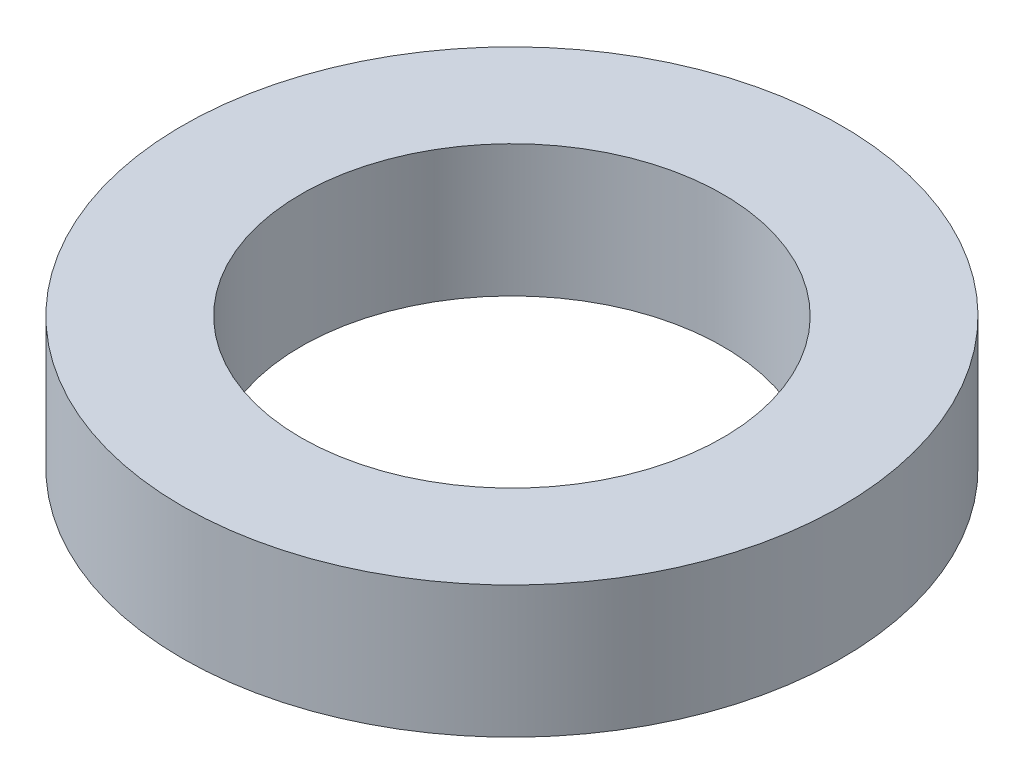
ISO-10303-21;
HEADER;
FILE_DESCRIPTION(('STEP AP214'),'2;1');
FILE_NAME('part.step','',(''),(''),'','','');
FILE_SCHEMA(('AUTOMOTIVE_DESIGN { 1 0 10303 214 1 1 1 1 }'));
ENDSEC;
DATA;
#1=APPLICATION_CONTEXT('core data for automotive mechanical design processes');
#2=APPLICATION_PROTOCOL_DEFINITION('international standard','automotive_design',2000,#1);
#3=PRODUCT_CONTEXT('',#1,'mechanical');
#4=PRODUCT('Part','Part','',(#3));
#5=PRODUCT_RELATED_PRODUCT_CATEGORY('part','',(#4));
#6=PRODUCT_DEFINITION_FORMATION('','',#4);
#7=PRODUCT_DEFINITION_CONTEXT('part definition',#1,'design');
#8=PRODUCT_DEFINITION('design','',#6,#7);
#9=PRODUCT_DEFINITION_SHAPE('','',#8);
#10=(LENGTH_UNIT() NAMED_UNIT(*) SI_UNIT(.MILLI.,.METRE.));
#11=(NAMED_UNIT(*) PLANE_ANGLE_UNIT() SI_UNIT($,.RADIAN.));
#12=(NAMED_UNIT(*) SI_UNIT($,.STERADIAN.) SOLID_ANGLE_UNIT());
#13=UNCERTAINTY_MEASURE_WITH_UNIT(LENGTH_MEASURE(1.E-05),#10,'distance_accuracy_value','');
#14=(GEOMETRIC_REPRESENTATION_CONTEXT(3) GLOBAL_UNCERTAINTY_ASSIGNED_CONTEXT((#13)) GLOBAL_UNIT_ASSIGNED_CONTEXT((#10,
#11,#12)) REPRESENTATION_CONTEXT('',''));
#15=CARTESIAN_POINT('',(0.,0.,0.));
#16=DIRECTION('',(0.,0.,1.));
#17=DIRECTION('',(1.,0.,0.));
#18=AXIS2_PLACEMENT_3D('',#15,#16,#17);
#19=CARTESIAN_POINT('',(0.,10.,0.));
#20=DIRECTION('',(0.,1.,0.));
#21=DIRECTION('',(0.,0.,1.));
#22=AXIS2_PLACEMENT_3D('',#19,#20,#21);
#23=PLANE('',#22);
#24=CARTESIAN_POINT('',(0.,10.,0.));
#25=DIRECTION('',(0.,1.,0.));
#26=DIRECTION('',(0.,0.,1.));
#27=AXIS2_PLACEMENT_3D('',#24,#25,#26);
#28=CIRCLE('',#27,25.);
#29=CARTESIAN_POINT('',(0.,10.,25.));
#30=VERTEX_POINT('',#29);
#31=EDGE_CURVE('E10',#30,#30,#28,.T.);
#32=ORIENTED_EDGE('',*,*,#31,.T.);
#33=EDGE_LOOP('',(#32));
#34=FACE_BOUND('',#33,.T.);
#35=CARTESIAN_POINT('',(0.,10.,0.));
#36=DIRECTION('',(0.,1.,0.));
#37=DIRECTION('',(0.,0.,1.));
#38=AXIS2_PLACEMENT_3D('',#35,#36,#37);
#39=CIRCLE('',#38,16.);
#40=CARTESIAN_POINT('',(0.,10.,16.));
#41=VERTEX_POINT('',#40);
#42=EDGE_CURVE('E49',#41,#41,#39,.T.);
#43=ORIENTED_EDGE('',*,*,#42,.F.);
#44=EDGE_LOOP('',(#43));
#45=FACE_BOUND('',#44,.T.);
#46=ADVANCED_FACE('F39',(#34,#45),#23,.T.);
#47=CARTESIAN_POINT('',(0.,0.,0.));
#48=DIRECTION('',(0.,1.,0.));
#49=DIRECTION('',(0.,0.,1.));
#50=AXIS2_PLACEMENT_3D('',#47,#48,#49);
#51=PLANE('',#50);
#52=CARTESIAN_POINT('',(0.,0.,0.));
#53=DIRECTION('',(0.,1.,0.));
#54=DIRECTION('',(0.,0.,1.));
#55=AXIS2_PLACEMENT_3D('',#52,#53,#54);
#56=CIRCLE('',#55,25.);
#57=CARTESIAN_POINT('',(0.,0.,25.));
#58=VERTEX_POINT('',#57);
#59=EDGE_CURVE('E43',#58,#58,#56,.T.);
#60=ORIENTED_EDGE('',*,*,#59,.F.);
#61=EDGE_LOOP('',(#60));
#62=FACE_BOUND('',#61,.T.);
#63=CARTESIAN_POINT('',(0.,0.,0.));
#64=DIRECTION('',(0.,1.,0.));
#65=DIRECTION('',(0.,0.,1.));
#66=AXIS2_PLACEMENT_3D('',#63,#64,#65);
#67=CIRCLE('',#66,16.);
#68=CARTESIAN_POINT('',(0.,0.,16.));
#69=VERTEX_POINT('',#68);
#70=EDGE_CURVE('E55',#69,#69,#67,.T.);
#71=ORIENTED_EDGE('',*,*,#70,.T.);
#72=EDGE_LOOP('',(#71));
#73=FACE_BOUND('',#72,.T.);
#74=ADVANCED_FACE('F65',(#62,#73),#51,.F.);
#75=CARTESIAN_POINT('',(0.,10.,0.));
#76=DIRECTION('',(0.,-1.,0.));
#77=DIRECTION('',(0.,0.,-1.));
#78=AXIS2_PLACEMENT_3D('',#75,#76,#77);
#79=CYLINDRICAL_SURFACE('',#78,25.);
#80=ORIENTED_EDGE('',*,*,#31,.F.);
#81=EDGE_LOOP('',(#80));
#82=FACE_BOUND('',#81,.T.);
#83=ORIENTED_EDGE('',*,*,#59,.T.);
#84=EDGE_LOOP('',(#83));
#85=FACE_BOUND('',#84,.T.);
#86=ADVANCED_FACE('F41',(#82,#85),#79,.T.);
#87=CARTESIAN_POINT('',(0.,10.,0.));
#88=DIRECTION('',(0.,-1.,0.));
#89=DIRECTION('',(0.,0.,-1.));
#90=AXIS2_PLACEMENT_3D('',#87,#88,#89);
#91=CYLINDRICAL_SURFACE('',#90,16.);
#92=ORIENTED_EDGE('',*,*,#42,.T.);
#93=EDGE_LOOP('',(#92));
#94=FACE_BOUND('',#93,.T.);
#95=ORIENTED_EDGE('',*,*,#70,.F.);
#96=EDGE_LOOP('',(#95));
#97=FACE_BOUND('',#96,.T.);
#98=ADVANCED_FACE('F59',(#94,#97),#91,.F.);
#99=CLOSED_SHELL('',(#46,#74,#86,#98));
#100=MANIFOLD_SOLID_BREP('B2',#99);
#101=ADVANCED_BREP_SHAPE_REPRESENTATION('',(#18,#100),#14);
#102=SHAPE_DEFINITION_REPRESENTATION(#9,#101);
ENDSEC;
END-ISO-10303-21;
